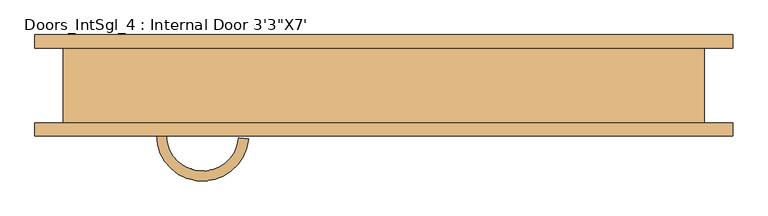
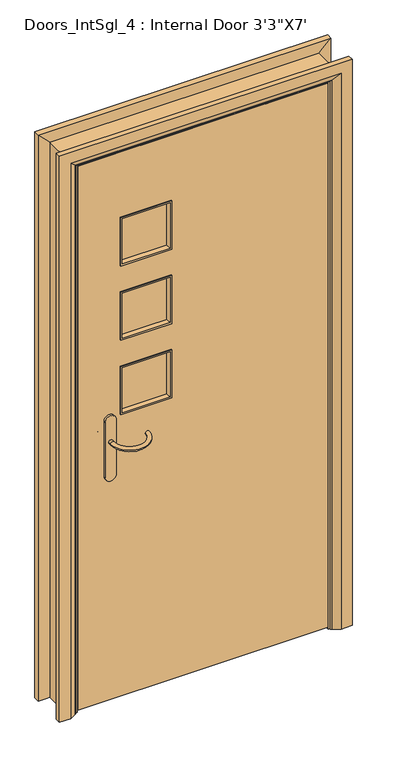
"""IFC4 building model written with IfcOpenShell, lengths in millimetres: door geometry."""

from ifc_helpers import new_model, si_unit, point, frame, frame_2d, origin, place, context, project, spatial, polyline, circle_curve, ellipse_curve, trimmed, segment, composite_curve, outline, extrude, faceted_brep, source, transform, mapped, element, save
from ifc_brep_helpers import plane_surface, cylinder_surface, revolved_surface, advanced_brep


def door_181986ca(model_context):
    return source(origin(), model_context, "Body", "SolidModel", [
        advanced_brep(
        [(-345.5, -11.15, 1000.0), (-330.5, -11.15, 1000.0), (-345.5, -1.15, 1000.0), (-330.5, -1.15, 1000.0), (-205.5986682, 4.9582241, 1000.0), (-220.5415886, 3.6508879, 1000.0)],
        [
            (0, 1, circle_curve(frame((-338.0, -11.15, 1000.0), z_axis=(0.0, -1.0, 0.0), x_axis=(1.0, 0.0, 0.0)), 7.5)),
            (1, 0, circle_curve(frame((-338.0, -11.15, 1000.0), z_axis=(0.0, -1.0, 0.0), x_axis=(1.0, 0.0, 0.0)), 7.5)),
            (0, 2),
            (2, 3, circle_curve(frame((-338.0, -1.15, 1000.0), z_axis=(0.0, -1.0, 0.0), x_axis=(1.0, 0.0, 0.0)), 7.5)),
            (3, 1),
            (3, 2, circle_curve(frame((-338.0, -1.15, 1000.0), z_axis=(0.0, -1.0, 0.0), x_axis=(1.0, 0.0, 0.0)), 7.5)),
            (4, 5, circle_curve(frame((-213.0701284, 4.304556, 1000.0), z_axis=(0.08715574274766678, -0.9961946980917448, 0.0), x_axis=(-0.9961946980917448, -0.08715574274766678, 0.0)), 7.5)),
            (5, 4, circle_curve(frame((-213.0701284, 4.304556, 1000.0), z_axis=(0.08715574274766678, -0.9961946980917448, 0.0), x_axis=(-0.9961946980917448, -0.08715574274766678, 0.0)), 7.5)),
            (5, 3, circle_curve(frame((-275.4159887, -1.15, 1000.0), z_axis=(0.0, 0.0, 1.0), x_axis=(-1.0, 0.0, 0.0)), 55.0840113)),
            (2, 4, circle_curve(frame((-275.4159887, -1.15, 1000.0), z_axis=(0.0, 0.0, -1.0), x_axis=(-1.0, 0.0, 0.0)), 70.0840113)),
        ],
        [
            plane_surface(frame((-338.0, -11.15, 1000.0), z_axis=(0.0, -1.0, 0.0), x_axis=(0.0, 0.0, 1.0))),
            cylinder_surface(frame((-338.0, -11.15, 1000.0), z_axis=(0.0, -1.0, 0.0), x_axis=(1.0, 0.0, 0.0)), 7.5),
            plane_surface(frame((-213.0701284, 4.304556, 1000.0), z_axis=(0.08715574274766678, -0.9961946980917448, 0.0), x_axis=(0.0, 0.0, 1.0))),
            revolved_surface(trimmed(ellipse_curve(frame((-338.0, -1.15, 1000.0), z_axis=(0.0, -1.0, 0.0), x_axis=(1.0, 0.0, 0.0)), 7.5, 7.5), [point((-345.5, -1.15, 1000.0))], [point((-330.5, -1.15, 1000.0))], True, "CARTESIAN"), (-275.4159887, -1.15, 1000.0), (0.0, 0.0, -1.0)),
            revolved_surface(trimmed(ellipse_curve(frame((-338.0, -1.15, 1000.0), z_axis=(0.0, -1.0, 0.0), x_axis=(1.0, 0.0, 0.0)), 7.5, 7.5), [point((-330.5, -1.15, 1000.0))], [point((-345.5, -1.15, 1000.0))], True, "CARTESIAN"), (-275.4159887, -1.15, 1000.0), (0.0, 0.0, -1.0)),
        ],
        [
            (0, [[1, 2]]),
            (1, [[-1, 3, 4, 5]]),
            (1, [[-2, -5, 6, -3]]),
            (2, [[7, 8]]),
            (3, [[9, -4, 10, -8]]),
            (4, [[-10, -6, -9, -7]]),
        ],
    ),
        extrude(outline(composite_curve([segment(trimmed(circle_curve(frame_2d((870.0, -338.0)), 20.0), [point((870.0, -358.0))], [point((870.0, -318.0))], False, "CARTESIAN"), True, "CONTINUOUS"), segment(polyline([(870.0, -318.0), (1080.0, -318.0)]), True, "CONTINUOUS"), segment(trimmed(circle_curve(frame_2d((1080.0, -338.0)), 20.0), [point((1080.0, -318.0))], [point((1080.0, -358.0))], False, "CARTESIAN"), True, "CONTINUOUS"), segment(polyline([(1080.0, -358.0), (870.0, -358.0)]), True, "CONTINUOUS")], self_intersect=False)), frame((0.0, -19.15, 0.0), z_axis=(0.0, 1.0, 0.0), x_axis=(0.0, 0.0, 1.0)), (0.0, 0.0, 1.0), 8.0),
        advanced_brep(
        [(-345.5, -65.15, 1000.0), (-330.5, -65.15, 1000.0), (-330.5, -75.15, 1000.0), (-345.5, -75.15, 1000.0), (-205.5986682, -81.2582241, 1000.0), (-220.5415886, -79.9508879, 1000.0)],
        [
            (0, 1, circle_curve(frame((-338.0, -65.15, 1000.0), z_axis=(0.0, 1.0, 0.0), x_axis=(1.0, 0.0, 0.0)), 7.5)),
            (1, 0, circle_curve(frame((-338.0, -65.15, 1000.0), z_axis=(0.0, 1.0, 0.0), x_axis=(1.0, 0.0, 0.0)), 7.5)),
            (1, 2),
            (2, 3, circle_curve(frame((-338.0, -75.15, 1000.0), z_axis=(0.0, 1.0, 0.0), x_axis=(1.0, 0.0, 0.0)), 7.5)),
            (3, 0),
            (3, 2, circle_curve(frame((-338.0, -75.15, 1000.0), z_axis=(0.0, 1.0, 0.0), x_axis=(1.0, 0.0, 0.0)), 7.5)),
            (4, 5, circle_curve(frame((-213.0701284, -80.604556, 1000.0), z_axis=(0.08715574274766356, 0.9961946980917451, 0.0), x_axis=(-0.9961946980917451, 0.08715574274766356, 0.0)), 7.5)),
            (5, 4, circle_curve(frame((-213.0701284, -80.604556, 1000.0), z_axis=(0.08715574274766356, 0.9961946980917451, 0.0), x_axis=(-0.9961946980917451, 0.08715574274766356, 0.0)), 7.5)),
            (4, 3, circle_curve(frame((-275.4159887, -75.15, 1000.0), z_axis=(0.0, 0.0, -1.0), x_axis=(-1.0, 0.0, 0.0)), 70.0840113)),
            (2, 5, circle_curve(frame((-275.4159887, -75.15, 1000.0), z_axis=(0.0, 0.0, 1.0), x_axis=(-1.0, 0.0, 0.0)), 55.0840113)),
        ],
        [
            plane_surface(frame((-338.0, -65.15, 1000.0), z_axis=(0.0, 1.0, 0.0), x_axis=(0.0, 0.0, 1.0))),
            cylinder_surface(frame((-338.0, -65.15, 1000.0), z_axis=(0.0, 1.0, 0.0), x_axis=(1.0, 0.0, 0.0)), 7.5),
            plane_surface(frame((-213.0701284, -80.604556, 1000.0), z_axis=(0.08715574274766356, 0.9961946980917451, 0.0), x_axis=(0.0, 0.0, 1.0))),
            revolved_surface(trimmed(ellipse_curve(frame((-338.0, -75.15, 1000.0), z_axis=(0.0, -1.0, 0.0), x_axis=(1.0, 0.0, 0.0)), 7.5, 7.5), [point((-345.5, -75.15, 1000.0))], [point((-330.5, -75.15, 1000.0))], True, "CARTESIAN"), (-275.4159887, -75.15, 1000.0), (0.0, 0.0, -1.0)),
            revolved_surface(trimmed(ellipse_curve(frame((-338.0, -75.15, 1000.0), z_axis=(0.0, -1.0, 0.0), x_axis=(1.0, 0.0, 0.0)), 7.5, 7.5), [point((-330.5, -75.15, 1000.0))], [point((-345.5, -75.15, 1000.0))], True, "CARTESIAN"), (-275.4159887, -75.15, 1000.0), (0.0, 0.0, -1.0)),
        ],
        [
            (0, [[1, 2]]),
            (1, [[3, 4, 5, -2]]),
            (1, [[-5, 6, -3, -1]]),
            (2, [[7, 8]]),
            (3, [[-7, 9, -4, 10]]),
            (4, [[-8, -10, -6, -9]]),
        ],
    ),
        extrude(outline(composite_curve([segment(trimmed(circle_curve(frame_2d((870.0, -338.0)), 20.0), [point((870.0, -358.0))], [point((870.0, -318.0))], False, "CARTESIAN"), True, "CONTINUOUS"), segment(polyline([(870.0, -318.0), (1080.0, -318.0)]), True, "CONTINUOUS"), segment(trimmed(circle_curve(frame_2d((1080.0, -338.0)), 20.0), [point((1080.0, -318.0))], [point((1080.0, -358.0))], False, "CARTESIAN"), True, "CONTINUOUS"), segment(polyline([(1080.0, -358.0), (870.0, -358.0)]), True, "CONTINUOUS")], self_intersect=False)), frame((0.0, -65.15, 0.0), z_axis=(0.0, 1.0, 0.0), x_axis=(0.0, 0.0, 1.0)), (0.0, 0.0, 1.0), 8.0),
        extrude(outline(polyline([(2091.6, -453.3), (8.0, -453.3), (8.0, 453.3), (2091.6, 453.3), (2091.6, -453.3)]), holes=[polyline([(1841.6, -113.3), (1656.6, -113.3), (1656.6, -298.3), (1841.6, -298.3), (1841.6, -113.3)]), polyline([(1086.6, -298.3), (1271.6, -298.3), (1271.6, -113.3), (1086.6, -113.3), (1086.6, -298.3)]), polyline([(1556.6, -113.3), (1371.6, -113.3), (1371.6, -298.3), (1556.6, -298.3), (1556.6, -113.3)])]), frame((0.0, -57.15, 0.0), z_axis=(0.0, 1.0, 0.0), x_axis=(0.0, 0.0, 1.0)), (0.0, 0.0, 1.0), 38.0),
        faceted_brep([(-455.3, -57.15, 0.0), (-487.3, -57.15, 0.0), (-487.3, 57.15, 0.0), (-455.3, 57.15, 0.0), (-455.3, 57.15, 2093.6), (-455.3, -57.15, 2093.6), (-487.3, 57.15, 2125.6), (-487.3, -57.15, 2125.6), (455.3, -57.15, 0.0), (455.3, 57.15, 0.0), (487.3, 57.15, 0.0), (487.3, -57.15, 0.0), (455.3, -57.15, 2093.6), (487.3, -57.15, 2125.6), (487.3, 57.15, 2125.6), (455.3, 57.15, 2093.6)], [[[0, 1, 2, 3]], [[3, 4, 5, 0]], [[2, 6, 4, 3]], [[1, 7, 6, 2]], [[0, 5, 7, 1]], [[8, 9, 10, 11]], [[12, 8, 11, 13]], [[13, 11, 10, 14]], [[14, 10, 9, 15]], [[15, 9, 8, 12]], [[4, 15, 12, 5]], [[6, 14, 15, 4]], [[7, 13, 14, 6]], [[5, 12, 13, 7]]]),
        advanced_brep(
        [(-530.3, 77.15, 0.0), (-490.3, 77.15, 0.0), (-464.3, 63.15, 0.0), (-460.3, 57.15, 0.0), (-530.3, 57.15, 0.0), (-530.3, 57.15, 2168.6), (-530.3, 77.15, 2168.6), (-460.3, 57.15, 2098.6), (-464.3, 63.15, 2102.6), (-490.3, 77.15, 2128.6), (530.3, 77.15, 0.0), (530.3, 57.15, 0.0), (460.3, 57.15, 0.0), (464.3, 63.15, 0.0), (490.3, 77.15, 0.0), (530.3, 77.15, 2168.6), (490.3, 77.15, 2128.6), (464.3, 63.15, 2102.6), (460.3, 57.15, 2098.6), (530.3, 57.15, 2168.6)],
        [
            (0, 1),
            (1, 2),
            (2, 3, circle_curve(frame((-468.3, 56.15, 0.0), z_axis=(0.0, 0.0, -1.0), x_axis=(-1.0, 0.0, 0.0)), 8.0622577)),
            (3, 4),
            (4, 0),
            (4, 5),
            (5, 6),
            (6, 0),
            (3, 7),
            (7, 5),
            (2, 8),
            (8, 7, ellipse_curve(frame((-468.3, 56.15, 2106.6), z_axis=(-0.7071067811865475, 0.0, -0.7071067811865475), x_axis=(0.7071067811865474, 0.0, -0.7071067811865476)), 11.4017543, 8.0622577)),
            (1, 9),
            (9, 8),
            (6, 9),
            (10, 11),
            (11, 12),
            (12, 13, circle_curve(frame((468.3, 56.15, 0.0), z_axis=(0.0, 0.0, -1.0), x_axis=(1.0, 0.0, 0.0)), 8.0622577)),
            (13, 14),
            (14, 10),
            (15, 10),
            (14, 16),
            (16, 15),
            (13, 17),
            (17, 16),
            (12, 18),
            (18, 17, ellipse_curve(frame((468.3, 56.15, 2106.6), z_axis=(0.7071067811865475, 0.0, -0.7071067811865475), x_axis=(0.7071067811865474, 0.0, 0.7071067811865476)), 11.4017543, 8.0622577)),
            (11, 19),
            (19, 18),
            (15, 19),
            (5, 19),
            (15, 6),
            (7, 18),
            (8, 17),
            (9, 16),
        ],
        [
            plane_surface(frame((-460.3, 129.9510989, 0.0), z_axis=(0.0, 0.0, -1.0), x_axis=(1.0, 0.0, 0.0))),
            plane_surface(frame((-530.3, 77.15, 0.0), z_axis=(-1.0, 0.0, 0.0), x_axis=(0.0, 0.0, 1.0))),
            plane_surface(frame((-530.3, 57.15, 0.0), z_axis=(0.0, -1.0, 0.0), x_axis=(0.0, 0.0, 1.0))),
            cylinder_surface(frame((-468.3, 56.15, 0.0), z_axis=(0.0, 0.0, -1.0), x_axis=(-1.0, 0.0, 0.0)), 8.0622577),
            plane_surface(frame((-464.3, 63.15, 0.0), z_axis=(0.4740998230350183, 0.8804710999221749, 0.0), x_axis=(0.0, 0.0, 1.0))),
            plane_surface(frame((-490.3, 77.15, 0.0), z_axis=(0.0, 1.0, 0.0), x_axis=(0.0, 0.0, 1.0))),
            plane_surface(frame((460.3, 129.9510989, 0.0), z_axis=(0.0, 0.0, -1.0), x_axis=(-1.0, 0.0, 0.0))),
            plane_surface(frame((490.3, 77.15, 2128.6), z_axis=(0.0, 1.0, 0.0), x_axis=(0.0, 0.0, -1.0))),
            plane_surface(frame((464.3, 63.15, 2102.6), z_axis=(-0.4740998230350183, 0.8804710999221749, 0.0), x_axis=(0.0, 0.0, -1.0))),
            cylinder_surface(frame((468.3, 56.15, 2098.6), z_axis=(0.0, 0.0, 1.0), x_axis=(1.0, 0.0, 0.0)), 8.0622577),
            plane_surface(frame((530.3, 57.15, 2168.6), z_axis=(0.0, -1.0, 0.0), x_axis=(0.0, 0.0, -1.0))),
            plane_surface(frame((530.3, 77.15, 2168.6), z_axis=(1.0, 0.0, 0.0), x_axis=(0.0, 0.0, -1.0))),
            plane_surface(frame((-530.3, 77.15, 2168.6), z_axis=(0.0, 0.0, 1.0), x_axis=(1.0, 0.0, 0.0))),
            plane_surface(frame((-530.3, 57.15, 2168.6), z_axis=(0.0, -1.0, 0.0), x_axis=(1.0, 0.0, 0.0))),
            cylinder_surface(frame((-460.3, 56.15, 2106.6), z_axis=(-1.0, 0.0, 0.0), x_axis=(0.0, 0.0, 1.0)), 8.0622577),
            plane_surface(frame((-464.3, 63.15, 2102.6), z_axis=(0.0, 0.8804710999221749, -0.4740998230350183), x_axis=(1.0, 0.0, 0.0))),
            plane_surface(frame((-490.3, 77.15, 2128.6), z_axis=(0.0, 1.0, 0.0), x_axis=(1.0, 0.0, 0.0))),
        ],
        [
            (0, [[1, 2, 3, 4, 5]]),
            (1, [[6, 7, 8, -5]]),
            (2, [[9, 10, -6, -4]]),
            (3, [[11, 12, -9, -3]]),
            (4, [[13, 14, -11, -2]]),
            (5, [[-8, 15, -13, -1]]),
            (6, [[16, 17, 18, 19, 20]]),
            (7, [[21, -20, 22, 23]]),
            (8, [[-22, -19, 24, 25]]),
            (9, [[-24, -18, 26, 27]]),
            (10, [[-26, -17, 28, 29]]),
            (11, [[-28, -16, -21, 30]]),
            (12, [[31, -30, 32, -7]]),
            (13, [[33, -29, -31, -10]]),
            (14, [[34, -27, -33, -12]]),
            (15, [[35, -25, -34, -14]]),
            (16, [[-32, -23, -35, -15]]),
        ],
    ),
        extrude(outline(polyline([(0.0, -436.3), (2074.6, -436.3), (2074.6, 436.3), (0.0, 436.3), (0.0, 455.3), (2093.6, 455.3), (2093.6, -455.3), (0.0, -455.3), (0.0, -436.3)])), frame((0.0, -17.15, 0.0), z_axis=(0.0, 1.0, 0.0), x_axis=(0.0, 0.0, 1.0)), (0.0, 0.0, 1.0), 32.0),
        advanced_brep(
        [(530.3, -77.15, 0.0), (490.3, -77.15, 0.0), (464.3, -63.15, 0.0), (460.3, -57.15, 0.0), (530.3, -57.15, 0.0), (530.3, -57.15, 2168.6), (530.3, -77.15, 2168.6), (460.3, -57.15, 2098.6), (-460.3, -57.15, 2098.6), (-460.3, -57.15, 0.0), (-530.3, -57.15, 0.0), (-530.3, -57.15, 2168.6), (464.3, -63.15, 2102.6), (490.3, -77.15, 2128.6), (-530.3, -77.15, 2168.6), (-530.3, -77.15, 0.0), (-490.3, -77.15, 0.0), (-490.3, -77.15, 2128.6), (-464.3, -63.15, 0.0), (-464.3, -63.15, 2102.6)],
        [
            (0, 1),
            (1, 2),
            (2, 3, circle_curve(frame((468.3, -56.15, 0.0), z_axis=(0.0, 0.0, -1.0), x_axis=(1.0, 0.0, 0.0)), 8.0622577)),
            (3, 4),
            (4, 0),
            (4, 5),
            (5, 6),
            (6, 0),
            (3, 7),
            (7, 8),
            (8, 9),
            (9, 10),
            (10, 11),
            (11, 5),
            (2, 12),
            (12, 7, ellipse_curve(frame((468.3, -56.15, 2106.6), z_axis=(0.7071067811865475, 0.0, -0.7071067811865475), x_axis=(-0.7071067811865474, 0.0, -0.7071067811865476)), 11.4017543, 8.0622577)),
            (1, 13),
            (13, 12),
            (6, 14),
            (14, 15),
            (15, 16),
            (16, 17),
            (17, 13),
            (10, 15),
            (14, 11),
            (9, 18, circle_curve(frame((-468.3, -56.15, 0.0), z_axis=(0.0, 0.0, -1.0), x_axis=(-1.0, 0.0, 0.0)), 8.0622577)),
            (18, 16),
            (19, 18),
            (8, 19, ellipse_curve(frame((-468.3, -56.15, 2106.6), z_axis=(-0.7071067811865475, 0.0, -0.7071067811865475), x_axis=(-0.7071067811865474, 0.0, 0.7071067811865476)), 11.4017543, 8.0622577)),
            (19, 17),
            (12, 19),
        ],
        [
            plane_surface(frame((460.3, -57.15, 0.0), z_axis=(0.0, 0.0, -1.0), x_axis=(0.0, 1.0, 0.0))),
            plane_surface(frame((530.3, -77.15, 0.0), z_axis=(1.0, 0.0, 0.0), x_axis=(0.0, 0.0, 1.0))),
            plane_surface(frame((530.3, -57.15, 0.0), z_axis=(0.0, 1.0, 0.0), x_axis=(0.0, 0.0, 1.0))),
            cylinder_surface(frame((468.3, -56.15, 0.0), z_axis=(0.0, 0.0, -1.0), x_axis=(1.0, 0.0, 0.0)), 8.0622577),
            plane_surface(frame((464.3, -63.15, 0.0), z_axis=(-0.4740998230350126, -0.8804710999221779, 0.0), x_axis=(0.0, 0.0, 1.0))),
            plane_surface(frame((490.3, -77.15, 0.0), z_axis=(0.0, -1.0, 0.0), x_axis=(0.0, 0.0, 1.0))),
            plane_surface(frame((-530.3, -77.15, 2168.6), z_axis=(-1.0, 0.0, 0.0), x_axis=(0.0, 0.0, -1.0))),
            plane_surface(frame((-460.3, -57.15, 0.0), z_axis=(0.0, 0.0, -1.0), x_axis=(0.0, 1.0, 0.0))),
            cylinder_surface(frame((-468.3, -56.15, 2098.6), z_axis=(0.0, 0.0, 1.0), x_axis=(-1.0, 0.0, 0.0)), 8.0622577),
            plane_surface(frame((-464.3, -63.15, 2102.6), z_axis=(0.4740998230350183, -0.8804710999221749, 0.0), x_axis=(0.0, 0.0, -1.0))),
            plane_surface(frame((530.3, -77.15, 2168.6), z_axis=(0.0, 0.0, 1.0), x_axis=(-1.0, 0.0, 0.0))),
            cylinder_surface(frame((460.3, -56.15, 2106.6), z_axis=(1.0, 0.0, 0.0), x_axis=(0.0, 0.0, 1.0)), 8.0622577),
            plane_surface(frame((464.3, -63.15, 2102.6), z_axis=(0.0, -0.8804710999221763, -0.4740998230350154), x_axis=(-1.0, 0.0, 0.0))),
        ],
        [
            (0, [[1, 2, 3, 4, 5]]),
            (1, [[6, 7, 8, -5]]),
            (2, [[9, 10, 11, 12, 13, 14, -6, -4]]),
            (3, [[15, 16, -9, -3]]),
            (4, [[17, 18, -15, -2]]),
            (5, [[-8, 19, 20, 21, 22, 23, -17, -1]]),
            (6, [[-13, 24, -20, 25]]),
            (7, [[-24, -12, 26, 27, -21]]),
            (8, [[28, -26, -11, 29]]),
            (9, [[-22, -27, -28, 30]]),
            (10, [[-14, -25, -19, -7]]),
            (11, [[31, -29, -10, -16]]),
            (12, [[-23, -30, -31, -18]]),
        ],
    ),
        faceted_brep([(-113.3, -60.15, 1841.6), (-113.3, -60.15, 1656.6), (-113.3, -47.15, 1656.6), (-113.3, -47.15, 1841.6), (-125.3, -47.15, 1829.6), (-125.3, -47.15, 1668.6), (-119.3, -60.15, 1662.6), (-119.3, -60.15, 1835.6), (-298.3, -60.15, 1656.6), (-298.3, -47.15, 1656.6), (-286.3, -47.15, 1668.6), (-292.3, -60.15, 1662.6), (-298.3, -60.15, 1841.6), (-298.3, -47.15, 1841.6), (-286.3, -47.15, 1829.6), (-292.3, -60.15, 1835.6)], [[[0, 1, 2, 3]], [[4, 5, 6, 7]], [[1, 8, 9, 2]], [[5, 10, 11, 6]], [[8, 12, 13, 9]], [[10, 14, 15, 11]], [[3, 2, 9, 13], [5, 4, 14, 10]], [[12, 0, 3, 13]], [[1, 0, 12, 8], [7, 6, 11, 15]], [[14, 4, 7, 15]]]),
        faceted_brep([(-119.3, -16.15, 1835.6), (-119.3, -16.15, 1662.6), (-125.3, -29.15, 1668.6), (-125.3, -29.15, 1829.6), (-113.3, -29.15, 1841.6), (-113.3, -29.15, 1656.6), (-113.3, -16.15, 1656.6), (-113.3, -16.15, 1841.6), (-292.3, -16.15, 1662.6), (-286.3, -29.15, 1668.6), (-298.3, -29.15, 1656.6), (-298.3, -16.15, 1656.6), (-292.3, -16.15, 1835.6), (-286.3, -29.15, 1829.6), (-298.3, -29.15, 1841.6), (-298.3, -16.15, 1841.6)], [[[0, 1, 2, 3]], [[4, 5, 6, 7]], [[1, 8, 9, 2]], [[5, 10, 11, 6]], [[8, 12, 13, 9]], [[10, 14, 15, 11]], [[12, 0, 3, 13]], [[7, 6, 11, 15], [1, 0, 12, 8]], [[14, 4, 7, 15]], [[5, 4, 14, 10], [3, 2, 9, 13]]]),
        extrude(outline(polyline([(-298.3, -47.15), (-298.3, -29.15), (-113.3, -29.15), (-113.3, -47.15), (-298.3, -47.15)])), frame((0.0, 0.0, 1656.6), z_axis=(0.0, 0.0, 1.0), x_axis=(1.0, 0.0, 0.0)), (0.0, 0.0, 1.0), 185.0),
        extrude(outline(polyline([(-298.3, -47.15), (-298.3, -29.15), (-113.3, -29.15), (-113.3, -47.15), (-298.3, -47.15)])), frame((0.0, 0.0, 1086.6), z_axis=(0.0, 0.0, 1.0), x_axis=(1.0, 0.0, 0.0)), (0.0, 0.0, 1.0), 185.0),
        extrude(outline(polyline([(-298.3, -47.15), (-298.3, -29.15), (-113.3, -29.15), (-113.3, -47.15), (-298.3, -47.15)])), frame((0.0, 0.0, 1371.6), z_axis=(0.0, 0.0, 1.0), x_axis=(1.0, 0.0, 0.0)), (0.0, 0.0, 1.0), 185.0),
        faceted_brep([(-298.3, -60.15, 1371.6), (-298.3, -60.15, 1556.6), (-298.3, -47.15, 1556.6), (-298.3, -47.15, 1371.6), (-286.3, -47.15, 1383.6), (-286.3, -47.15, 1544.6), (-292.3, -60.15, 1550.6), (-292.3, -60.15, 1377.6), (-113.3, -60.15, 1556.6), (-113.3, -47.15, 1556.6), (-125.3, -47.15, 1544.6), (-119.3, -60.15, 1550.6), (-113.3, -60.15, 1371.6), (-113.3, -47.15, 1371.6), (-125.3, -47.15, 1383.6), (-119.3, -60.15, 1377.6)], [[[0, 1, 2, 3]], [[4, 5, 6, 7]], [[1, 8, 9, 2]], [[5, 10, 11, 6]], [[8, 12, 13, 9]], [[10, 14, 15, 11]], [[3, 2, 9, 13], [5, 4, 14, 10]], [[12, 0, 3, 13]], [[1, 0, 12, 8], [7, 6, 11, 15]], [[14, 4, 7, 15]]]),
        faceted_brep([(-298.3, -60.15, 1086.6), (-298.3, -60.15, 1271.6), (-298.3, -47.15, 1271.6), (-298.3, -47.15, 1086.6), (-286.3, -47.15, 1098.6), (-286.3, -47.15, 1259.6), (-292.3, -60.15, 1265.6), (-292.3, -60.15, 1092.6), (-113.3, -60.15, 1271.6), (-113.3, -47.15, 1271.6), (-125.3, -47.15, 1259.6), (-119.3, -60.15, 1265.6), (-113.3, -60.15, 1086.6), (-113.3, -47.15, 1086.6), (-125.3, -47.15, 1098.6), (-119.3, -60.15, 1092.6)], [[[0, 1, 2, 3]], [[4, 5, 6, 7]], [[1, 8, 9, 2]], [[5, 10, 11, 6]], [[8, 12, 13, 9]], [[10, 14, 15, 11]], [[3, 2, 9, 13], [5, 4, 14, 10]], [[12, 0, 3, 13]], [[1, 0, 12, 8], [7, 6, 11, 15]], [[14, 4, 7, 15]]]),
        faceted_brep([(-113.3, -16.15, 1371.6), (-113.3, -16.15, 1556.6), (-113.3, -29.15, 1556.6), (-113.3, -29.15, 1371.6), (-125.3, -29.15, 1383.6), (-125.3, -29.15, 1544.6), (-119.3, -16.15, 1550.6), (-119.3, -16.15, 1377.6), (-298.3, -16.15, 1556.6), (-298.3, -29.15, 1556.6), (-286.3, -29.15, 1544.6), (-292.3, -16.15, 1550.6), (-298.3, -16.15, 1371.6), (-298.3, -29.15, 1371.6), (-286.3, -29.15, 1383.6), (-292.3, -16.15, 1377.6)], [[[0, 1, 2, 3]], [[4, 5, 6, 7]], [[1, 8, 9, 2]], [[5, 10, 11, 6]], [[8, 12, 13, 9]], [[10, 14, 15, 11]], [[3, 2, 9, 13], [5, 4, 14, 10]], [[12, 0, 3, 13]], [[1, 0, 12, 8], [7, 6, 11, 15]], [[14, 4, 7, 15]]]),
        faceted_brep([(-113.3, -16.15, 1086.6), (-113.3, -16.15, 1271.6), (-113.3, -29.15, 1271.6), (-113.3, -29.15, 1086.6), (-125.3, -29.15, 1098.6), (-125.3, -29.15, 1259.6), (-119.3, -16.15, 1265.6), (-119.3, -16.15, 1092.6), (-298.3, -16.15, 1271.6), (-298.3, -29.15, 1271.6), (-286.3, -29.15, 1259.6), (-292.3, -16.15, 1265.6), (-298.3, -16.15, 1086.6), (-298.3, -29.15, 1086.6), (-286.3, -29.15, 1098.6), (-292.3, -16.15, 1092.6)], [[[0, 1, 2, 3]], [[4, 5, 6, 7]], [[1, 8, 9, 2]], [[5, 10, 11, 6]], [[8, 12, 13, 9]], [[10, 14, 15, 11]], [[3, 2, 9, 13], [5, 4, 14, 10]], [[12, 0, 3, 13]], [[1, 0, 12, 8], [7, 6, 11, 15]], [[14, 4, 7, 15]]]),
    ])


if __name__ == "__main__":
    model = new_model("IFC4")
    model_context = context("Model", 3, world=origin())
    ifc_project = project(units=[si_unit("LENGTHUNIT", "METRE", prefix="MILLI")], contexts=[model_context])
    site = spatial("IfcSite", under=ifc_project)
    building = spatial("IfcBuilding", under=site)
    placement = place(None, origin())
    door_shape = door_181986ca(model_context)
    element("IfcDoor", 1, ObjectType="Doors_IntSgl_4 : Internal Door 3'3\"X7'", at=placement, inside=building, context=model_context, shape_type="MappedRepresentation", body=[
        mapped(door_shape, transform((0.0, 0.0, 0.0), x_axis=(1.0, 0.0, 0.0), y_axis=(0.0, 1.0, 0.0), z_axis=(0.0, 0.0, 1.0))),
    ])
    save(model, "model.ifc")

# Revit data of these elements
# Type "Doors_IntSgl_4 : Internal Door 3'3\"X7'"
#   Type Mark = "13"
#   Type Comments = "Internal Single"
#   Operation = "SingleSwingRight"
#   Construction Type Id = "SGL"
#   Manufacturer = "Revit"
#   Keynote = "L20"
#   Description = "Internal Single Door"
#   Analytic Construction = "Large single-glazed windows"
#   Visual Light Transmittance = 0.9
#   VisionPanel Width = 0' - 7.28346"
#   VisionPanel Depth = 0' - 7.28346"
#   UnderCut = 0' - 0.31496"
#   Tolerance = 0' - 0.07874"
#   Thickness = 0' - 1.49606"
#   Structural Tolerance = 0' - 0.31496"
#   StopDepth = 0' - 1.25984"
#   Stop Thickness = 0' - 0.74803"
#   Stile Shutting = 0' - 6.10236"
#   Stile Top Rail = 0' - 9.84252"
#   Stile Intermediate/Frieze = 0' - 3.93701"
#   Solar Heat Gain Coefficient = 0.86
#   Rough Width = 3' - 3"
#   Rough Height = 7' - 0"
#   Heat Transfer Coefficient (U) = 0.979472 BTU/(h·ft²·°F)
#   Handle Z Distance = 3' - 3.37008"
#   Handle X Distance = 0' - 2.95276"
#   Handle Length = 1' - 1.77953"
#   Frame Thickness = 0' - 1.25984"
#   Door Panel Width = 2' - 11.69291"
#   Door Panel Thickness = 0' - 1.49606"
#   Door Panel Offset = 0' - 0"
#   Height = 7' - 0"
#   Width = 3' - 3"
#   Door Panel Height = 6' - 10.0315"
#   Architrave Setback = 0' - 0.19685"
#   Vis - Ironmongery = yes
#   Define Thermal Properties by = 1
#   Material Ironmongery = Door - Handle
#   Material Glass = Door - Glazing
#   Material Frame = Door - Frame/Mullion
#   Material Door = Door - Panel
#   Material Beading = Door - Panel
#   Material Architrave = Door - Architrave
#   Handle Style = element 386699
#   Function = (empty or 0)
#   Wall Closure = (empty or 0)
# Element 1 (IfcDoor, "Doors_IntSgl_4 : Internal Door 3'3\"X7'")
#   Materials on its faces: "Door - Panel", "Door - Architrave", "Door - Handle", "Door - Frame/Mullion", "Door - Glazing"
# Materials
#   "Door - Handle": colour RGB 247 247 247, transparency 0
#   "Door - Glazing": colour RGB 0 0 255, transparency 0.75
#   "Door - Frame/Mullion": class "Wood", colour RGB 212 179 113, transparency 0
#   "Door - Panel": class "Wood", colour RGB 210 159 95, transparency 0, Cost = 0
#   "Door - Architrave": class "Wood", colour RGB 212 179 113, transparency 0
